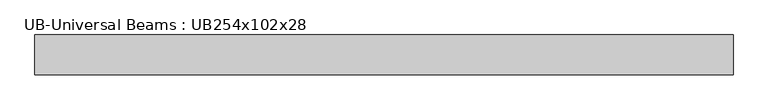
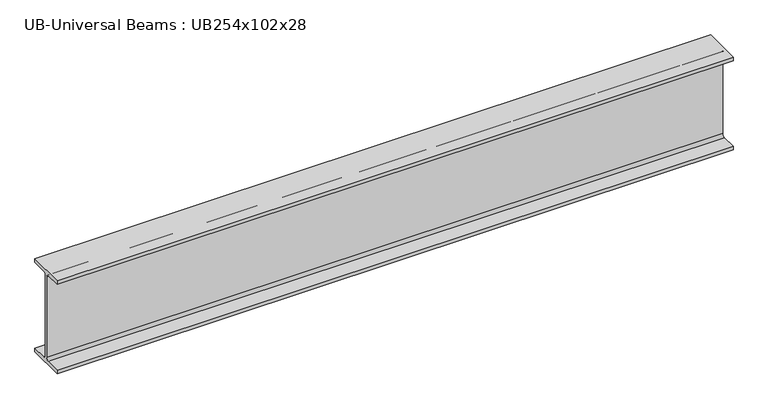
"""IFC4 building model written with IfcOpenShell, lengths in millimetres: beam geometry, UB-Universal Beams : UB254x102x28."""

from ifc_helpers import new_model, si_unit, point, frame, frame_2d, origin, place, context, project, spatial, polyline, circle_curve, trimmed, segment, composite_curve, outline, extrude, source, transform, mapped, element, save


def ub_universal_beams_ub254x102x28_3582687b(model_context):
    return source(origin(), model_context, "Body", "SweptSolid", [
        extrude(outline(composite_curve([segment(polyline([(51.1, -120.2), (51.1, -130.2), (-51.1, -130.2), (-51.1, -120.2), (-10.75, -120.2)]), True, "CONTINUOUS"), segment(trimmed(circle_curve(frame_2d((-10.75, -112.6)), 7.6), [point((-10.75, -120.2))], [point((-3.15, -112.6))], True, "CARTESIAN"), True, "CONTINUOUS"), segment(polyline([(-3.15, -112.6), (-3.15, 112.6)]), True, "CONTINUOUS"), segment(trimmed(circle_curve(frame_2d((-10.75, 112.6)), 7.6), [point((-3.15, 112.6))], [point((-10.75, 120.2))], True, "CARTESIAN"), True, "CONTINUOUS"), segment(polyline([(-10.75, 120.2), (-51.1, 120.2), (-51.1, 130.2), (51.1, 130.2), (51.1, 120.2), (10.75, 120.2)]), True, "CONTINUOUS"), segment(trimmed(circle_curve(frame_2d((10.75, 112.6)), 7.6), [point((10.75, 120.2))], [point((3.15, 112.6))], True, "CARTESIAN"), True, "CONTINUOUS"), segment(polyline([(3.15, 112.6), (3.15, -112.6)]), True, "CONTINUOUS"), segment(trimmed(circle_curve(frame_2d((10.75, -112.6)), 7.6), [point((3.15, -112.6))], [point((10.75, -120.2))], True, "CARTESIAN"), True, "CONTINUOUS"), segment(polyline([(10.75, -120.2), (51.1, -120.2)]), True, "CONTINUOUS")], self_intersect=False)), frame((-1016.0, 0.0, 0.0), z_axis=(1.0, 0.0, 0.0), x_axis=(0.0, 1.0, 0.0)), (0.0, 0.0, 1.0), 1793.1),
    ])


if __name__ == "__main__":
    model = new_model("IFC4")
    model_context = context("Model", 3, world=origin())
    ifc_project = project(units=[si_unit("LENGTHUNIT", "METRE", prefix="MILLI")], contexts=[model_context])
    site = spatial("IfcSite", under=ifc_project)
    building = spatial("IfcBuilding", under=site)
    placement = place(None, origin())
    ub_universal_beams_ub254x102x28_shape = ub_universal_beams_ub254x102x28_3582687b(model_context)
    element("IfcBeam", 1, ObjectType="UB-Universal Beams : UB254x102x28", at=placement, inside=building, context=model_context, shape_type="MappedRepresentation", body=[
        mapped(ub_universal_beams_ub254x102x28_shape, transform((0.0, 0.0, 0.0), x_axis=(1.0, 0.0, 0.0), y_axis=(0.0, 1.0, 0.0), z_axis=(0.0, 0.0, 1.0))),
    ])
    save(model, "model.ifc")

# Revit data of these elements
# Type "UB-Universal Beams : UB254x102x28"
#   Section Name Key = "UB254X102X28"
#   Width = 10.22 cm
#   Web Thickness = 0.63 cm
#   Web Fillet = 0.76 cm
#   Warping Constant = 28000.0 cm⁶
#   Torsional Moment of Inertia = 9.57 cm⁴
#   Section Area = 36.1 cm²
#   Plastic Modulus weak axis = 54.8 cm³
#   Plastic Modulus strong axis = 353.0 cm³
#   Nominal Weight = 28.2999 kgf/m
#   Moment of Inertia weak axis = 179.00 cm⁴
#   Moment of Inertia strong axis = 4005.00 cm⁴
#   Height = 26.04 cm
#   Flange Thickness = 1.0 cm
#   Elastic Modulus weak axis = 34.9 cm³
#   Elastic Modulus strong axis = 308.0 cm³
#   Centroid Vertical = 13.02 cm
#   Centroid Horizontal = 5.11 cm
#   Bolt Spacing = 5.4 cm
#   Length [instance default] = 4' - 11.05512"
#   Structural Material [instance default] = Metal - Steel 43-275
#   Type Comments = ""
#   Assembly Code = ""
# Element 1 (IfcBeam, "UB-Universal Beams : UB254x102x28")
#   Materials on its faces: "Metal - Steel 43-275"
# Materials
#   "Metal - Steel 43-275": class "Metal", colour RGB 247 247 247, transparency 0, Cost = 0
